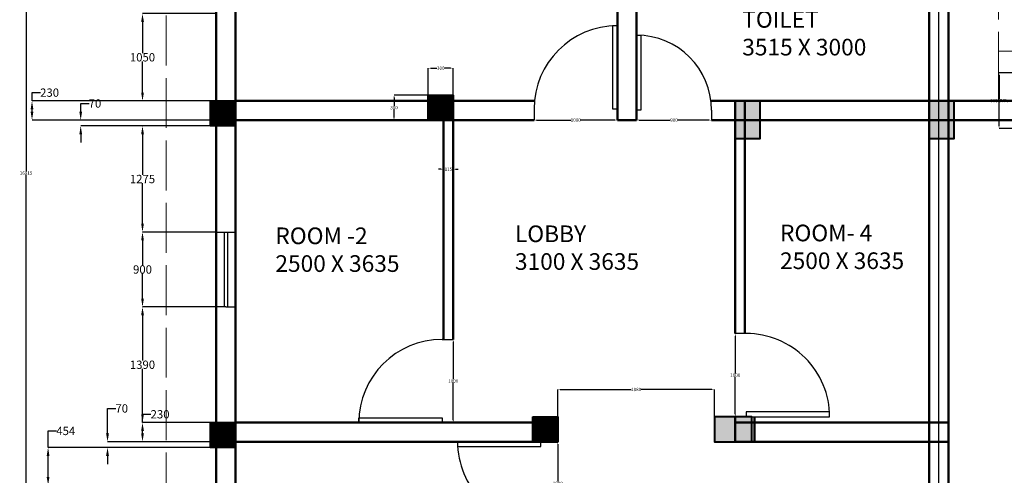
# Model space of a CAD drawing. Units: millimetres. Extents: x -17156 to 39375, y -45872 to -24892.
# Tile 2 of 12: x -17156 to -5337, y -39337 to -33861. Entities that reach past the tile are written whole.
import ezdxf

# ---------------------------------------------------------------- set-up
doc = ezdxf.new("R2010")
doc.units = ezdxf.units.MM
doc.header["$MEASUREMENT"] = 0
doc.linetypes.add('ACAD_ISO02W100', pattern=[15, 12, -3])
for name, color, linetype, lineweight in [('A-ANNO-DIMS', 2, 'Continuous', 18), ('A-AREA-IDEN', 4, 'Continuous', 25), ('A-COLS', 7, 'Continuous', 40), ('A-ROOF', 8, 'Continuous', 18), ('A-ROOF-OVHD', 8, 'ACAD_ISO02W100', 18), ('DOORS', 6, 'Continuous', 25), ('WALLS', 5, 'Continuous', 50), ('WINDOW', 240, 'Continuous', 25)]:
    doc.layers.add(name, color=color, linetype=linetype, lineweight=lineweight)
doc.styles.get("Standard").update_dxf_attribs({"font": 'arial.ttf'})
doc.dimstyles.get("Standard").update_dxf_attribs({"dimtxt": 40, "dimasz": 30.18, "dimexe": 0, "dimexo": 0.0625, "dimgap": 0.09, "dimtad": 0, "dimtih": 1, "dimtoh": 1, "dimdec": 0, "dimzin": 0, "dimdsep": 46, "dimtxsty": 'Standard', "dimcen": 0.09, "dimadec": 0, "dimazin": 0, "dimtfac": 1, "dimtdec": 0, "dimtofl": 0, "dimtmove": 0, "dimatfit": 3, "dimfxl": 1, "dimtolj": 1, "dimtzin": 0, "dimarcsym": 0})

# ---------------------------------------------------------------- blocks, each defined once
blk = doc.blocks.new('*U5')
for p, q in [((0, 0), (0, -100)), ((750, 0), (750, -100))]:
    blk.add_line(p, q)
blk.add_lwpolyline([(0, 0), (0, 750), (43.75, 750), (43.75, 0)], close=True)
blk.add_arc((0, 0), 750, 0, 90)
blk = doc.blocks.new('*U3')
for p, q in [((-750, 0), (-750, -100)), ((0, 0), (0, -100))]:
    blk.add_line(p, q)
blk.add_lwpolyline([(0, 0), (0, 750), (-43.75, 750), (-43.75, 0)], close=True)
blk.add_arc((0, 0), 750, 90, 180)
blk = doc.blocks.new('*U6')
for p, q in [((-750, 0), (-750, 100)), ((0, 0), (0, 100))]:
    blk.add_line(p, q)
blk.add_lwpolyline([(0, 0), (0, -750), (-43.75, -750), (-43.75, 0)], close=True)
blk.add_arc((0, 0), 750, 180, 270)
blk = doc.blocks.new('*U7')
for p, q in [((0, 0), (0, 100)), ((750, 0), (750, 100))]:
    blk.add_line(p, q)
blk.add_lwpolyline([(0, 0), (0, -750), (43.75, -750), (43.75, 0)], close=True)
blk.add_arc((0, 0), 750, 270, 0)
blk = doc.blocks.new('*D15')
at = {"layer": 'A-ANNO-DIMS', "color": 0, "lineweight": -2, "transparency": 16777216}
for p, q in [((-16815, -39003), (-16815, -38803)), ((-16815, -38803), (-16715, -38803)), ((-14867, -39003), (-16815, -39003)), ((-16815, -39357), (-16815, -39103)), ((-14797, -39457), (-16815, -39457))]:
    blk.add_line(p, q, dxfattribs=at)
at = {"layer": 'A-ANNO-DIMS', "color": 0, "lineweight": 100, "transparency": 16777216}
for points in [[(-16832, -39103), (-16799, -39103), (-16815, -39003)], [(-16832, -39357), (-16799, -39357), (-16815, -39457)]]:
    blk.add_solid(points, dxfattribs=at)
at = {"layer": 'Defpoints', "color": 0, "lineweight": 100, "transparency": 16777216}
for p in [(-16815, -39003), (-14867, -39003), (-14797, -39457)]:
    blk.add_point(p, dxfattribs=at)
at = {"layer": 'A-ANNO-DIMS', "color": 0, "transparency": 16777216, "insert": (-16603, -38803), "char_height": 100, "attachment_point": 5}
blk.add_mtext('\\A1;454', dxfattribs=at)
blk = doc.blocks.new('*D16')
at = {"layer": 'A-ANNO-DIMS', "color": 0, "lineweight": -2, "transparency": 16777216}
for p, q in [((-16102, -38833), (-16102, -38533)), ((-16102, -38533), (-16002, -38533)), ((-14567, -38933), (-16102, -38933)), ((-14867, -39003), (-16102, -39003)), ((-16102, -39103), (-16102, -39203))]:
    blk.add_line(p, q, dxfattribs=at)
at = {"layer": 'A-ANNO-DIMS', "color": 0, "lineweight": 100, "transparency": 16777216}
for points in [[(-16119, -38833), (-16085, -38833), (-16102, -38933)], [(-16119, -39103), (-16085, -39103), (-16102, -39003)]]:
    blk.add_solid(points, dxfattribs=at)
at = {"layer": 'Defpoints', "color": 0, "lineweight": 100, "transparency": 16777216}
for p in [(-16102, -38933), (-14567, -38933), (-14867, -39003)]:
    blk.add_point(p, dxfattribs=at)
at = {"layer": 'A-ANNO-DIMS', "color": 0, "transparency": 16777216, "insert": (-15931, -38533), "char_height": 100, "attachment_point": 5}
blk.add_mtext('\\A1;70', dxfattribs=at)
blk = doc.blocks.new('*D17')
at = {"layer": 'A-ANNO-DIMS', "color": 0, "lineweight": -2, "transparency": 16777216}
for p, q in [((-15682, -38703), (-15682, -38603)), ((-15682, -38603), (-15582, -38603)), ((-14867, -38703), (-15682, -38703)), ((-15682, -38833), (-15682, -38803)), ((-14567, -38933), (-15682, -38933))]:
    blk.add_line(p, q, dxfattribs=at)
at = {"layer": 'A-ANNO-DIMS', "color": 0, "lineweight": 100, "transparency": 16777216}
for points in [[(-15698, -38803), (-15665, -38803), (-15682, -38703)], [(-15698, -38833), (-15665, -38833), (-15682, -38933)]]:
    blk.add_solid(points, dxfattribs=at)
at = {"layer": 'Defpoints', "color": 0, "lineweight": 100, "transparency": 16777216}
for p in [(-15682, -38703), (-14867, -38703), (-14567, -38933)]:
    blk.add_point(p, dxfattribs=at)
at = {"layer": 'A-ANNO-DIMS', "color": 0, "transparency": 16777216, "insert": (-15471, -38603), "char_height": 100, "attachment_point": 5}
blk.add_mtext('\\A1;230', dxfattribs=at)
blk = doc.blocks.new('*D18')
at = {"layer": 'A-ANNO-DIMS', "color": 0, "lineweight": -2, "transparency": 16777216}
for p, q in [((-14797, -37313), (-15682, -37313)), ((-15682, -37413), (-15682, -37957)), ((-15682, -38603), (-15682, -38059)), ((-14867, -38703), (-15682, -38703))]:
    blk.add_line(p, q, dxfattribs=at)
at = {"layer": 'A-ANNO-DIMS', "color": 0, "lineweight": 100, "transparency": 16777216}
for points in [[(-15698, -37413), (-15665, -37413), (-15682, -37313)], [(-15698, -38603), (-15665, -38603), (-15682, -38703)]]:
    blk.add_solid(points, dxfattribs=at)
at = {"layer": 'Defpoints', "color": 0, "lineweight": 100, "transparency": 16777216}
for p in [(-15682, -37313), (-14797, -37313), (-14867, -38703)]:
    blk.add_point(p, dxfattribs=at)
at = {"layer": 'A-ANNO-DIMS', "color": 0, "transparency": 16777216, "insert": (-15682, -38008), "char_height": 100, "attachment_point": 5}
blk.add_mtext('\\A1;1390', dxfattribs=at)
blk = doc.blocks.new('*D19')
at = {"layer": 'A-ANNO-DIMS', "color": 0, "lineweight": -2, "transparency": 16777216}
for p, q in [((-14797, -36413), (-15682, -36413)), ((-15682, -36513), (-15682, -36812)), ((-15682, -37213), (-15682, -36914)), ((-14797, -37313), (-15682, -37313))]:
    blk.add_line(p, q, dxfattribs=at)
at = {"layer": 'A-ANNO-DIMS', "color": 0, "lineweight": 100, "transparency": 16777216}
for points in [[(-15698, -36513), (-15665, -36513), (-15682, -36413)], [(-15698, -37213), (-15665, -37213), (-15682, -37313)]]:
    blk.add_solid(points, dxfattribs=at)
at = {"layer": 'Defpoints', "color": 0, "lineweight": 100, "transparency": 16777216}
for p in [(-15682, -36413), (-14797, -36413), (-14797, -37313)]:
    blk.add_point(p, dxfattribs=at)
at = {"layer": 'A-ANNO-DIMS', "color": 0, "transparency": 16777216, "insert": (-15682, -36863), "char_height": 100, "attachment_point": 5}
blk.add_mtext('\\A1;900', dxfattribs=at)
blk = doc.blocks.new('*D20')
at = {"layer": 'A-ANNO-DIMS', "color": 0, "lineweight": -2, "transparency": 16777216}
for p, q in [((-14867, -35138), (-15682, -35138)), ((-15682, -35238), (-15682, -35724)), ((-15682, -36313), (-15682, -35827)), ((-14797, -36413), (-15682, -36413))]:
    blk.add_line(p, q, dxfattribs=at)
at = {"layer": 'A-ANNO-DIMS', "color": 0, "lineweight": 100, "transparency": 16777216}
for points in [[(-15698, -35238), (-15665, -35238), (-15682, -35138)], [(-15698, -36313), (-15665, -36313), (-15682, -36413)]]:
    blk.add_solid(points, dxfattribs=at)
at = {"layer": 'Defpoints', "color": 0, "lineweight": 100, "transparency": 16777216}
for p in [(-15682, -35138), (-14867, -35138), (-14797, -36413)]:
    blk.add_point(p, dxfattribs=at)
at = {"layer": 'A-ANNO-DIMS', "color": 0, "transparency": 16777216, "insert": (-15682, -35776), "char_height": 100, "attachment_point": 5}
blk.add_mtext('\\A1;1275', dxfattribs=at)
blk = doc.blocks.new('*D21')
at = {"layer": 'A-ANNO-DIMS', "color": 0, "lineweight": -2, "transparency": 16777216}
for p, q in [((-16424, -34968), (-16424, -34868)), ((-16424, -34868), (-16324, -34868)), ((-14567, -35068), (-16424, -35068)), ((-14867, -35138), (-16424, -35138)), ((-16424, -35238), (-16424, -35338))]:
    blk.add_line(p, q, dxfattribs=at)
at = {"layer": 'A-ANNO-DIMS', "color": 0, "lineweight": 100, "transparency": 16777216}
for points in [[(-16440, -34968), (-16407, -34968), (-16424, -35068)], [(-16440, -35238), (-16407, -35238), (-16424, -35138)]]:
    blk.add_solid(points, dxfattribs=at)
at = {"layer": 'Defpoints', "color": 0, "lineweight": 100, "transparency": 16777216}
for p in [(-16424, -35068), (-14567, -35068), (-14867, -35138)]:
    blk.add_point(p, dxfattribs=at)
at = {"layer": 'A-ANNO-DIMS', "color": 0, "transparency": 16777216, "insert": (-16253, -34868), "char_height": 100, "attachment_point": 5}
blk.add_mtext('\\A1;70', dxfattribs=at)
blk = doc.blocks.new('*D22')
at = {"layer": 'A-ANNO-DIMS', "color": 0, "lineweight": -2, "transparency": 16777216}
for p, q in [((-17008, -34838), (-17008, -34738)), ((-17008, -34738), (-16908, -34738)), ((-14867, -34838), (-17008, -34838)), ((-17008, -34968), (-17008, -34938)), ((-14567, -35068), (-17008, -35068))]:
    blk.add_line(p, q, dxfattribs=at)
at = {"layer": 'A-ANNO-DIMS', "color": 0, "lineweight": 100, "transparency": 16777216}
for points in [[(-17025, -34938), (-16992, -34938), (-17008, -34838)], [(-17025, -34968), (-16992, -34968), (-17008, -35068)]]:
    blk.add_solid(points, dxfattribs=at)
at = {"layer": 'Defpoints', "color": 0, "lineweight": 100, "transparency": 16777216}
for p in [(-17008, -34838), (-14867, -34838), (-14567, -35068)]:
    blk.add_point(p, dxfattribs=at)
at = {"layer": 'A-ANNO-DIMS', "color": 0, "transparency": 16777216, "insert": (-16797, -34738), "char_height": 100, "attachment_point": 5}
blk.add_mtext('\\A1;230', dxfattribs=at)
blk = doc.blocks.new('*D23')
at = {"layer": 'A-ANNO-DIMS', "color": 0, "lineweight": -2, "transparency": 16777216}
for p, q in [((-14797, -33788), (-15682, -33788)), ((-15682, -33888), (-15682, -34262)), ((-15682, -34738), (-15682, -34364)), ((-14867, -34838), (-15682, -34838))]:
    blk.add_line(p, q, dxfattribs=at)
at = {"layer": 'A-ANNO-DIMS', "color": 0, "lineweight": 100, "transparency": 16777216}
for points in [[(-15698, -33888), (-15665, -33888), (-15682, -33788)], [(-15698, -34738), (-15665, -34738), (-15682, -34838)]]:
    blk.add_solid(points, dxfattribs=at)
at = {"layer": 'Defpoints', "color": 0, "lineweight": 100, "transparency": 16777216}
for p in [(-15682, -33788), (-14797, -33788), (-14867, -34838)]:
    blk.add_point(p, dxfattribs=at)
at = {"layer": 'A-ANNO-DIMS', "color": 0, "transparency": 16777216, "insert": (-15682, -34313), "char_height": 100, "attachment_point": 5}
blk.add_mtext('\\A1;1050', dxfattribs=at)
blk = doc.blocks.new('*D82')
at = {"layer": 'A-ANNO-DIMS', "color": 0, "lineweight": -2, "transparency": 16777216}
for p, q in [((-10982, -35068), (-10982, -35068)), ((-10952, -35068), (-10540, -35068)), ((-10013, -35068), (-10424, -35068)), ((-9982, -35068), (-9982, -35068))]:
    blk.add_line(p, q, dxfattribs=at)
at = {"layer": 'A-ANNO-DIMS', "color": 0, "lineweight": 100, "transparency": 16777216}
for points in [[(-10952, -35063), (-10952, -35073), (-10982, -35068)], [(-10013, -35063), (-10013, -35073), (-9982, -35068)]]:
    blk.add_solid(points, dxfattribs=at)
at = {"layer": 'Defpoints', "color": 0, "lineweight": 100, "transparency": 16777216}
for p in [(-10982, -35068), (-9982, -35068), (-9982, -35068)]:
    blk.add_point(p, dxfattribs=at)
at = {"layer": 'A-ANNO-DIMS', "color": 0, "transparency": 16777216, "insert": (-10482, -35068), "char_height": 40, "attachment_point": 5}
blk.add_mtext('\\A1;1000', dxfattribs=at)
blk = doc.blocks.new('*D83')
at = {"layer": 'A-ANNO-DIMS', "color": 0, "lineweight": -2, "transparency": 16777216}
for p, q in [((-9752, -35068), (-9752, -35068)), ((-9722, -35068), (-9347, -35068)), ((-8883, -35068), (-9258, -35068)), ((-8852, -35068), (-8852, -35068))]:
    blk.add_line(p, q, dxfattribs=at)
at = {"layer": 'A-ANNO-DIMS', "color": 0, "lineweight": 100, "transparency": 16777216}
for points in [[(-9722, -35063), (-9722, -35073), (-9752, -35068)], [(-8883, -35063), (-8883, -35073), (-8852, -35068)]]:
    blk.add_solid(points, dxfattribs=at)
at = {"layer": 'Defpoints', "color": 0, "lineweight": 100, "transparency": 16777216}
for p in [(-9752, -35068), (-8852, -35068), (-8852, -35068)]:
    blk.add_point(p, dxfattribs=at)
at = {"layer": 'A-ANNO-DIMS', "color": 0, "transparency": 16777216, "insert": (-9302, -35068), "char_height": 40, "attachment_point": 5}
blk.add_mtext('\\A1;900', dxfattribs=at)
blk = doc.blocks.new('*D84')
at = {"layer": 'A-ANNO-DIMS', "color": 0, "lineweight": -2, "transparency": 16777216}
for p, q in [((-12098, -35658), (-12128, -35658)), ((-12067, -35850), (-12067, -35658)), ((-11952, -35850), (-11952, -35658)), ((-11922, -35658), (-11892, -35658))]:
    blk.add_line(p, q, dxfattribs=at)
at = {"layer": 'A-ANNO-DIMS', "color": 0, "lineweight": 100, "transparency": 16777216}
for points in [[(-12098, -35653), (-12098, -35663), (-12067, -35658)], [(-11922, -35653), (-11922, -35663), (-11952, -35658)]]:
    blk.add_solid(points, dxfattribs=at)
at = {"layer": 'Defpoints', "color": 0, "lineweight": 100, "transparency": 16777216}
for p in [(-11952, -35658), (-12067, -35850), (-11952, -35850)]:
    blk.add_point(p, dxfattribs=at)
at = {"layer": 'A-ANNO-DIMS', "color": 0, "transparency": 16777216, "insert": (-12010, -35658), "char_height": 40, "attachment_point": 5}
blk.add_mtext('\\A1;115', dxfattribs=at)
blk = doc.blocks.new('*D85')
at = {"layer": 'A-ANNO-DIMS', "color": 0, "lineweight": -2, "transparency": 16777216}
for p, q in [((-11952, -37703), (-11952, -37703)), ((-11952, -37733), (-11952, -38182)), ((-11952, -38673), (-11952, -38223)), ((-11952, -38703), (-11952, -38703))]:
    blk.add_line(p, q, dxfattribs=at)
at = {"layer": 'A-ANNO-DIMS', "color": 0, "lineweight": 100, "transparency": 16777216}
for points in [[(-11957, -37733), (-11947, -37733), (-11952, -37703)], [(-11957, -38673), (-11947, -38673), (-11952, -38703)]]:
    blk.add_solid(points, dxfattribs=at)
at = {"layer": 'Defpoints', "color": 0, "lineweight": 100, "transparency": 16777216}
for p in [(-11952, -37703), (-11952, -38703), (-11952, -38703)]:
    blk.add_point(p, dxfattribs=at)
at = {"layer": 'A-ANNO-DIMS', "color": 0, "transparency": 16777216, "insert": (-11952, -38203), "char_height": 40, "attachment_point": 5}
blk.add_mtext('\\A1;1000', dxfattribs=at)
blk = doc.blocks.new('*D86')
at = {"layer": 'A-ANNO-DIMS', "color": 0, "lineweight": -2, "transparency": 16777216}
for p, q in [((-8567, -37633), (-8567, -37633)), ((-8567, -37663), (-8567, -38112)), ((-8567, -38603), (-8567, -38153)), ((-8567, -38633), (-8567, -38633))]:
    blk.add_line(p, q, dxfattribs=at)
at = {"layer": 'A-ANNO-DIMS', "color": 0, "lineweight": 100, "transparency": 16777216}
for points in [[(-8572, -37663), (-8562, -37663), (-8567, -37633)], [(-8572, -38603), (-8562, -38603), (-8567, -38633)]]:
    blk.add_solid(points, dxfattribs=at)
at = {"layer": 'Defpoints', "color": 0, "lineweight": 100, "transparency": 16777216}
for p in [(-8567, -37633), (-8567, -38633), (-8567, -38633)]:
    blk.add_point(p, dxfattribs=at)
at = {"layer": 'A-ANNO-DIMS', "color": 0, "transparency": 16777216, "insert": (-8567, -38133), "char_height": 40, "attachment_point": 5}
blk.add_mtext('\\A1;1000', dxfattribs=at)
blk = doc.blocks.new('*D87')
at = {"layer": 'A-ANNO-DIMS', "color": 0, "lineweight": -2, "transparency": 16777216}
for p, q in [((-10697, -38633), (-10697, -38305)), ((-10667, -38305), (-9815, -38305)), ((-8848, -38305), (-9699, -38305)), ((-8817, -38633), (-8817, -38305))]:
    blk.add_line(p, q, dxfattribs=at)
at = {"layer": 'A-ANNO-DIMS', "color": 0, "lineweight": 100, "transparency": 16777216}
for points in [[(-10667, -38300), (-10667, -38310), (-10697, -38305)], [(-8848, -38300), (-8848, -38310), (-8817, -38305)]]:
    blk.add_solid(points, dxfattribs=at)
at = {"layer": 'Defpoints', "color": 0, "lineweight": 100, "transparency": 16777216}
for p in [(-10697, -38305), (-10697, -38633), (-8817, -38633)]:
    blk.add_point(p, dxfattribs=at)
at = {"layer": 'A-ANNO-DIMS', "color": 0, "transparency": 16777216, "insert": (-9757, -38305), "char_height": 40, "attachment_point": 5}
blk.add_mtext('\\A1;1880', dxfattribs=at)
blk = doc.blocks.new('*D89')
at = {"layer": 'A-ANNO-DIMS', "color": 0, "lineweight": -2, "transparency": 16777216}
for p, q in [((-10697, -38933), (-10697, -38933)), ((-10697, -38963), (-10697, -39412)), ((-10697, -39903), (-10697, -39453)), ((-10767, -39933), (-10697, -39933))]:
    blk.add_line(p, q, dxfattribs=at)
at = {"layer": 'A-ANNO-DIMS', "color": 0, "lineweight": 100, "transparency": 16777216}
for points in [[(-10702, -38963), (-10692, -38963), (-10697, -38933)], [(-10702, -39903), (-10692, -39903), (-10697, -39933)]]:
    blk.add_solid(points, dxfattribs=at)
at = {"layer": 'Defpoints', "color": 0, "lineweight": 100, "transparency": 16777216}
for p in [(-10697, -38933), (-10697, -38933), (-10767, -39933)]:
    blk.add_point(p, dxfattribs=at)
at = {"layer": 'A-ANNO-DIMS', "color": 0, "transparency": 16777216, "insert": (-10697, -39433), "char_height": 40, "attachment_point": 5}
blk.add_mtext('\\A1;1000', dxfattribs=at)
blk = doc.blocks.new('*D116')
at = {"layer": 'A-ANNO-DIMS', "color": 0, "lineweight": -2, "transparency": 16777216}
for p, q in [((-12252, -34768), (-12252, -34444)), ((-12222, -34444), (-12147, -34444)), ((-11983, -34444), (-12058, -34444)), ((-11952, -34768), (-11952, -34444))]:
    blk.add_line(p, q, dxfattribs=at)
at = {"layer": 'A-ANNO-DIMS', "color": 0, "lineweight": 100, "transparency": 16777216}
for points in [[(-12222, -34439), (-12222, -34449), (-12252, -34444)], [(-11983, -34439), (-11983, -34449), (-11952, -34444)]]:
    blk.add_solid(points, dxfattribs=at)
at = {"layer": 'Defpoints', "color": 0, "lineweight": 100, "transparency": 16777216}
for p in [(-12252, -34444), (-12252, -34768), (-11952, -34768)]:
    blk.add_point(p, dxfattribs=at)
at = {"layer": 'A-ANNO-DIMS', "color": 0, "transparency": 16777216, "insert": (-12102, -34444), "char_height": 40, "attachment_point": 5}
blk.add_mtext('\\A1;300', dxfattribs=at)
blk = doc.blocks.new('*D117')
at = {"layer": 'A-ANNO-DIMS', "color": 0, "lineweight": -2, "transparency": 16777216}
for p, q in [((-12252, -34768), (-12663, -34768)), ((-12663, -34798), (-12663, -34897)), ((-12663, -35038), (-12663, -34938)), ((-12252, -35068), (-12663, -35068))]:
    blk.add_line(p, q, dxfattribs=at)
at = {"layer": 'A-ANNO-DIMS', "color": 0, "lineweight": 100, "transparency": 16777216}
for points in [[(-12668, -34798), (-12658, -34798), (-12663, -34768)], [(-12668, -35038), (-12658, -35038), (-12663, -35068)]]:
    blk.add_solid(points, dxfattribs=at)
at = {"layer": 'Defpoints', "color": 0, "lineweight": 100, "transparency": 16777216}
for p in [(-12252, -34768), (-12663, -35068), (-12252, -35068)]:
    blk.add_point(p, dxfattribs=at)
at = {"layer": 'A-ANNO-DIMS', "color": 0, "transparency": 16777216, "insert": (-12663, -34918), "char_height": 40, "attachment_point": 5}
blk.add_mtext('\\A1;300', dxfattribs=at)
blk = doc.blocks.new('WIN-900x230')
for p, q in [((0, 900), (230, 900)), ((95, 900), (95, 0)), ((135, 900), (135, 0)), ((115, 0), (0, 0)), ((115, 0), (230, 0))]:
    blk.add_line(p, q)
blk = doc.blocks.new('COL-300x300')
h = blk.add_hatch()
h.set_pattern_fill('ANSI31', color=256)
h.paths.add_polyline_path([(300, 300), (0, 300), (0, 0), (300, 0)])
blk.add_lwpolyline([(0, 300), (300, 300), (300, 0), (0, 0)], close=True)
blk = doc.blocks.new('COL-450x300')
h = blk.add_hatch(color=256)
h.dxf.hatch_style = 1
h.paths.add_polyline_path([(0, 300), (0, 0), (450, 0), (450, 300)])
blk.add_lwpolyline([(0, 300), (0, 0), (450, 0), (450, 300)], close=True)
blk = doc.blocks.new('*D141')
at = {"layer": 'A-ANNO-DIMS', "color": 0, "lineweight": -2, "transparency": 16777216}
for p, q in [((-5146, -34500), (-5401, -34500)), ((-5401, -34530), (-5401, -34813)), ((-5401, -35138), (-5401, -34854)), ((-5146, -35168), (-5401, -35168))]:
    blk.add_line(p, q, dxfattribs=at)
at = {"layer": 'A-ANNO-DIMS', "color": 0, "lineweight": 100, "transparency": 16777216}
for points in [[(-5406, -34530), (-5396, -34530), (-5401, -34500)], [(-5406, -35138), (-5396, -35138), (-5401, -35168)]]:
    blk.add_solid(points, dxfattribs=at)
at = {"layer": 'Defpoints', "color": 0, "lineweight": 100, "transparency": 16777216}
for p in [(-5401, -34500), (-5146, -34500), (-5146, -35168)]:
    blk.add_point(p, dxfattribs=at)
at = {"layer": 'A-ANNO-DIMS', "color": 0, "transparency": 16777216, "insert": (-5401, -34834), "char_height": 40, "attachment_point": 5}
blk.add_mtext('\\A1;668 TYP.', dxfattribs=at)
blk = doc.blocks.new('*D145')
at = {"layer": 'A-ANNO-DIMS', "color": 0, "lineweight": -2, "transparency": 16777216}
for p, q in [((-6237, -27248), (-17080, -27248)), ((-17080, -27278), (-17080, -35685)), ((-17080, -44133), (-17080, -35726)), ((-2887, -44163), (-17080, -44163))]:
    blk.add_line(p, q, dxfattribs=at)
at = {"layer": 'A-ANNO-DIMS', "color": 0, "lineweight": 100, "transparency": 16777216}
for points in [[(-17085, -27278), (-17075, -27278), (-17080, -27248)], [(-17085, -44133), (-17075, -44133), (-17080, -44163)]]:
    blk.add_solid(points, dxfattribs=at)
at = {"layer": 'Defpoints', "color": 0, "lineweight": 100, "transparency": 16777216}
for p in [(-6237, -27248), (-17080, -44163), (-2887, -44163)]:
    blk.add_point(p, dxfattribs=at)
at = {"layer": 'A-ANNO-DIMS', "color": 0, "transparency": 16777216, "insert": (-17080, -35705), "char_height": 40, "attachment_point": 5}
blk.add_mtext('\\A1;16915', dxfattribs=at)
blk = doc.blocks.new('*D151')
at = {"layer": 'A-ANNO-DIMS', "color": 0, "lineweight": -2, "transparency": 16777216}
for p, q in [((-6122, -42548), (-6122, -25565)), ((-6092, -25565), (-4413, -25565)), ((-2615, -25565), (-4294, -25565)), ((-2584, -42548), (-2584, -25565))]:
    blk.add_line(p, q, dxfattribs=at)
at = {"layer": 'A-ANNO-DIMS', "color": 0, "lineweight": 100, "transparency": 16777216}
for points in [[(-6092, -25560), (-6092, -25570), (-6122, -25565)], [(-2615, -25560), (-2615, -25570), (-2584, -25565)]]:
    blk.add_solid(points, dxfattribs=at)
at = {"layer": 'Defpoints', "color": 0, "lineweight": 100, "transparency": 16777216}
for p in [(-2584, -25565), (-6122, -42548), (-2584, -42548)]:
    blk.add_point(p, dxfattribs=at)
at = {"layer": 'A-ANNO-DIMS', "color": 0, "transparency": 16777216, "insert": (-4353, -25565), "char_height": 40, "attachment_point": 5}
blk.add_mtext('\\A1;3538', dxfattribs=at)

msp = doc.modelspace()

# ---------------------------------------------------------------- linework, layer by layer
at = {"layer": 'A-ROOF'}
for q in [(-5407.35, -34837.85), (-3184.35, -34237.85)]:
    msp.add_line((-5407.35, -34237.85), q, dxfattribs=at)
at = {"layer": 'A-ROOF-OVHD', "ltscale": 50}
for p, q in [((-15397.35, -42662.85), (-15397.35, -31007.85)), ((-5407.35, -31007.85), (-5407.35, -34237.85)), ((-4295.85, -34237.85), (-5407.35, -34237.85))]:
    msp.add_line(p, q, dxfattribs=at)
at = {"layer": 'WALLS'}
for p, q in [((-6007.35, -27247.85), (-6007.35, -40562.85)), ((-14797.35, -42662.85), (-14797.35, -31607.85)), ((-9982.35, -35067.85), (-9982.35, -31607.85)), ((-9752.35, -35067.85), (-9752.35, -31607.85)), ((-14567.35, -34837.85), (-14567.35, -31837.85)), ((-6237.35, -33152.85), (-6237.35, -40562.85)), ((-14567.35, -34837.85), (-10977.67, -34837.85)), ((-12067.35, -37702.85), (-12067.35, -34837.85)), ((-11952.35, -37702.85), (-11952.35, -34837.85)), ((-8859.1, -34837.85), (-5045.85, -34837.85)), ((-8567.35, -37632.85), (-8567.35, -34837.85)), ((-8452.35, -37632.85), (-8452.35, -34837.85)), ((-14567.35, -35067.85), (-10982.35, -35067.85)), ((-14567.35, -38702.85), (-14567.35, -35067.85)), ((-9982.35, -35067.85), (-9752.35, -35067.85)), ((-8852.35, -35067.85), (-5145.85, -35067.85)), ((-8567.35, -38932.85), (-8567.35, -38632.85)), ((-8337.35, -38932.85), (-8337.35, -38632.85)), ((-14567.35, -38702.85), (-10697.35, -38702.85)), ((-10997.35, -38932.85), (-10997.35, -38702.85)), ((-10767.35, -38932.85), (-10767.35, -38702.85)), ((-8567.35, -38702.85), (-6007.35, -38702.85)), ((-14567.35, -42432.85), (-14567.35, -38932.85)), ((-14567.35, -38932.85), (-10697.36, -38932.85)), ((-8567.35, -38932.85), (-6007.35, -38932.85))]:
    msp.add_line(p, q, dxfattribs=at)

# ---------------------------------------------------------------- block references
at = {"layer": 'A-COLS'}
for name, p in [('COL-300x300', (-14867.35, -35137.85)), ('COL-300x300', (-12252.35, -35067.85)), ('COL-300x300', (-10997.35, -38932.85)), ('COL-450x300', (-8817.35, -38932.85)), ('COL-300x300', (-14867.35, -39002.85))]:
    msp.add_blockref(name, p, dxfattribs=at)
at = {"layer": 'A-COLS', "rotation": 90.00000000000124}
for p in [(-8267.35, -35287.85), (-5937.35, -35287.85)]:
    msp.add_blockref('COL-450x300', p, dxfattribs=at)
at = {"layer": 'DOORS'}
for name, p, xscale, yscale, zscale in [('*U3', (-9982.35, -34934.51), 1.333333333333333, 1.333333333333333, 1.333333333333333), ('*U5', (-9752.35, -34947.85), 1.199999999999999, 1.199999999999999, 1.199999999999999)]:
    msp.add_blockref(name, p, dxfattribs=dict(at, xscale=xscale, yscale=yscale, zscale=zscale))
at = {"layer": 'DOORS', "xscale": 1.333333333333333, "yscale": 1.333333333333333, "zscale": 1.333333333333333}
for name, p, rotation in [('*U7', (-8434.02, -38632.85), 89.99999999999999), ('*U6', (-12085.68, -38702.85), 270), ('*U7', (-10900.68, -38932.85), 270)]:
    msp.add_blockref(name, p, dxfattribs=dict(at, rotation=rotation))
at = {"layer": 'WINDOW'}
msp.add_blockref('WIN-900x230', (-14797.35, -37313.16), dxfattribs=at)

# ---------------------------------------------------------------- texts
at = {"layer": 'A-AREA-IDEN', "char_height": 200, "attachment_point": 1}
for s, width, insert in [('{TOILET \\P3515 X 3000}', 1569.8583, (-8483.16, -33757.73)), ('{ROOM -2\\P2500 X 3635}', 2181.7854, (-14087, -36358.64)), ('{LOBBY\\P3100 X 3635}', 3420.1917, (-11211.23, -36334.17)), ('{ROOM- 4 \\P2500 X 3635}', 3010.3341, (-8029.52, -36324.53))]:
    msp.add_mtext_dynamic_manual_height_columns(s, width=width, gutter_width=1, heights=[0], dxfattribs=dict(at, insert=insert))

# ---------------------------------------------------------------- dimensions: what is measured, and where the dimension line sits
at = {"layer": 'A-ANNO-DIMS'}
for base, p1, p2, override, picture, middle in [((-2584.35, -25564.85), (-6122.35, -42547.85), (-2584.35, -42547.85), {"dimdec": 0, "dimlfac": 1, "dimrnd": 0, "dimzin": 0, "dimdsep": 46, "dimlunit": 2}, '*D151', (-4353.35, -25564.85)), ((-12252.35, -34443.71), (-11952.35, -34767.85), (-12252.35, -34767.85), {"dimclrd": 0, "dimclre": 0, "dimclrt": 0}, '*D116', (-12102.35, -34443.71)), ((-9982.35, -35067.85), (-10982.35, -35067.85), (-9982.35, -35067.85), {"dimclrd": 0, "dimclre": 0, "dimclrt": 0}, '*D82', (-10482.35, -35067.85)), ((-8852.35, -35067.85), (-9752.35, -35067.85), (-8852.35, -35067.85), {"dimclrd": 0, "dimclre": 0, "dimclrt": 0}, '*D83', (-9302.35, -35067.85)), ((-11952.35, -35657.58), (-12067.35, -35850.44), (-11952.35, -35850.44), {"dimclrd": 0, "dimclre": 0, "dimclrt": 0}, '*D84', (-12009.85, -35657.58))]:
    dim = msp.add_linear_dim(base=base, p1=p1, p2=p2, dimstyle='Standard', override=override, dxfattribs=at)
    dim.commit()
    dim.dimension.update_dxf_attribs({"geometry": picture, "text_midpoint": middle})
for base, p1, p2, angle, override, picture, middle in [((-17080.35, -44162.85), (-6237.35, -27247.85), (-2887.35, -44162.85), 90, {"dimdec": 0, "dimlfac": 1, "dimrnd": 0, "dimzin": 0, "dimdsep": 46, "dimlunit": 2}, '*D145', (-17080.35, -35705.35)), ((-15681.77, -33788.06), (-14867.35, -34837.85), (-14797.35, -33788.06), 270, {"dimtxt": 100, "dimasz": 100, "dimclrd": 0, "dimclre": 0, "dimclrt": 0}, '*D23', (-15681.77, -34312.95)), ((-17008.47, -34837.85), (-14567.35, -35067.85), (-14867.35, -34837.85), 270, {"dimtxt": 100, "dimasz": 100, "dimclrd": 0, "dimclre": 0, "dimclrt": 0}, '*D22', (-16797.23, -34737.85)), ((-16423.65, -35067.85), (-14867.35, -35137.85), (-14567.35, -35067.85), 270, {"dimtxt": 100, "dimasz": 100, "dimclrd": 0, "dimclre": 0, "dimclrt": 0}, '*D21', (-16252.52, -34867.85)), ((-12662.66, -35067.85), (-12252.35, -34767.85), (-12252.35, -35067.85), 90, {"dimclrd": 0, "dimclre": 0, "dimclrt": 0}, '*D117', (-12662.66, -34917.85)), ((-15681.77, -35137.85), (-14797.35, -36413.16), (-14867.35, -35137.85), 270, {"dimtxt": 100, "dimasz": 100, "dimclrd": 0, "dimclre": 0, "dimclrt": 0}, '*D20', (-15681.77, -35775.5)), ((-15681.77, -36413.16), (-14797.35, -37313.16), (-14797.35, -36413.16), 270, {"dimtxt": 100, "dimasz": 100, "dimclrd": 0, "dimclre": 0, "dimclrt": 0}, '*D19', (-15681.77, -36863.16)), ((-15681.77, -37313.16), (-14867.35, -38702.85), (-14797.35, -37313.16), 270, {"dimtxt": 100, "dimasz": 100, "dimclrd": 0, "dimclre": 0, "dimclrt": 0}, '*D18', (-15681.77, -38008)), ((-8567.35, -38632.85), (-8567.35, -37632.85), (-8567.35, -38632.85), 90, {"dimclrd": 0, "dimclre": 0, "dimclrt": 0}, '*D86', (-8567.35, -38132.85)), ((-11952.35, -38702.85), (-11952.35, -37702.85), (-11952.35, -38702.85), 90, {"dimclrd": 0, "dimclre": 0, "dimclrt": 0}, '*D85', (-11952.35, -38202.85)), ((-15681.77, -38702.85), (-14567.35, -38932.85), (-14867.35, -38702.85), 270, {"dimtxt": 100, "dimasz": 100, "dimclrd": 0, "dimclre": 0, "dimclrt": 0}, '*D17', (-15470.53, -38602.85)), ((-10697.36, -38932.85), (-10767.35, -39932.85), (-10697.35, -38932.85), 90, {"dimclrd": 0, "dimclre": 0, "dimclrt": 0}, '*D89', (-10697.36, -39432.85))]:
    dim = msp.add_linear_dim(base=base, p1=p1, p2=p2, angle=angle, dimstyle='Standard', override=override, dxfattribs=at)
    dim.commit()
    dim.dimension.update_dxf_attribs({"geometry": picture, "text_midpoint": middle})
dim = msp.add_linear_dim(base=(-5400.85, -34499.85), p1=(-5145.85, -35167.85), p2=(-5145.85, -34499.85), angle=90, text='<> TYP.', dimstyle='Standard', override={"dimdec": 0, "dimlfac": 1, "dimrnd": 0, "dimzin": 0, "dimdsep": 46, "dimlunit": 2}, dxfattribs=at)
dim.commit()
dim.dimension.update_dxf_attribs({"geometry": '*D141', "text_midpoint": (-5400.85, -34833.85)})
dim = msp.add_linear_dim(base=(-10697.35, -38305.16), p1=(-8817.35, -38632.85), p2=(-10697.35, -38632.85), dimstyle='Standard', override={"dimclrd": 0, "dimclre": 0, "dimclrt": 0}, dxfattribs=at)
dim.commit()
dim.dimension.update_dxf_attribs({"geometry": '*D87', "text_midpoint": (-9757.35, -38305.16), "dimtype": 160})
for base, p1, p2, picture, middle in [((-16102.02, -38932.85), (-14867.35, -39002.85), (-14567.35, -38932.85), '*D16', (-15930.89, -38532.85)), ((-16815.49, -39002.85), (-14797.35, -39456.9), (-14867.35, -39002.85), '*D15', (-16603.12, -38802.85))]:
    dim = msp.add_linear_dim(base=base, p1=p1, p2=p2, angle=270, dimstyle='Standard', override={"dimtxt": 100, "dimasz": 100, "dimclrd": 0, "dimclre": 0, "dimclrt": 0}, dxfattribs=at)
    dim.commit()
    dim.dimension.update_dxf_attribs({"geometry": picture, "text_midpoint": middle, "dimtype": 160})

doc.saveas('drawing.dxf')
